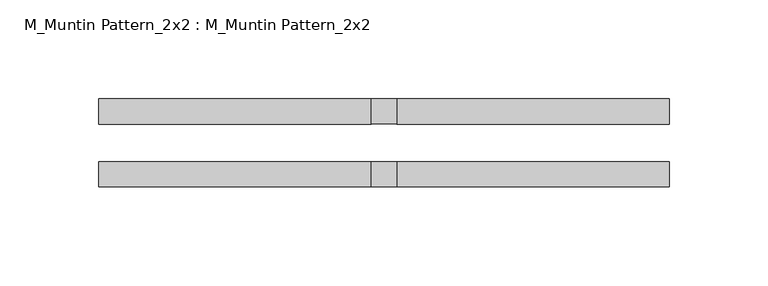
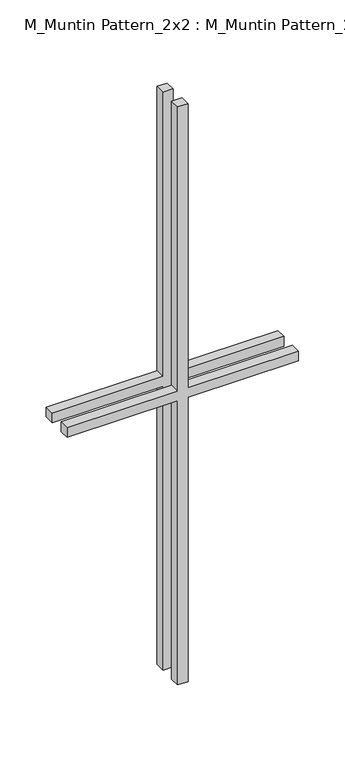
"""IFC4 building model written with IfcOpenShell, lengths in millimetres: proxy geometry, M_Muntin Pattern_2x2 : M_Muntin Pattern_2x2."""

from ifc_helpers import new_model, si_unit, frame, origin, place, context, project, spatial, polyline, outline, extrude, source, transform, mapped, element, save


def m_muntin_pattern_2x2_m_muntin_pattern_2x2_4fd78f17(model_context):
    return source(origin(), model_context, "Body", "SweptSolid", [
        extrude(outline(polyline([(386.5, -6.35), (386.5, -144.2375), (373.8, -144.2375), (373.8, -6.35), (0.0, -6.35), (0.0, 6.35), (373.8, 6.35), (373.8, 144.2375), (386.5, 144.2375), (386.5, 6.35), (760.3, 6.35), (760.3, -6.35), (386.5, -6.35)])), frame((0.0, -22.225, 0.0), z_axis=(0.0, 1.0, 0.0), x_axis=(0.0, 0.0, 1.0)), (0.0, 0.0, 1.0), 12.7),
        extrude(outline(polyline([(386.5, -6.35), (386.5, -144.2375), (373.8, -144.2375), (373.8, -6.35), (0.0, -6.35), (0.0, 6.35), (373.8, 6.35), (373.8, 144.2375), (386.5, 144.2375), (386.5, 6.35), (760.3, 6.35), (760.3, -6.35), (386.5, -6.35)])), frame((0.0, 9.525, 0.0), z_axis=(0.0, 1.0, 0.0), x_axis=(0.0, 0.0, 1.0)), (0.0, 0.0, 1.0), 12.7),
    ])


if __name__ == "__main__":
    model = new_model("IFC4")
    model_context = context("Model", 3, world=origin())
    ifc_project = project(units=[si_unit("LENGTHUNIT", "METRE", prefix="MILLI")], contexts=[model_context])
    site = spatial("IfcSite", under=ifc_project)
    building = spatial("IfcBuilding", under=site)
    placement = place(None, origin())
    m_muntin_pattern_2x2_m_muntin_pattern_2x2_shape = m_muntin_pattern_2x2_m_muntin_pattern_2x2_4fd78f17(model_context)
    element("IfcBuildingElementProxy", 1, Name="M_Muntin Pattern_2x2 : M_Muntin Pattern_2x2", ObjectType="M_Muntin Pattern_2x2 : M_Muntin Pattern_2x2", at=placement, inside=building, context=model_context, shape_type="MappedRepresentation", body=[
        mapped(m_muntin_pattern_2x2_m_muntin_pattern_2x2_shape, transform((0.0, 0.0, 0.0), x_axis=(1.0, 0.0, 0.0), y_axis=(0.0, 1.0, 0.0), z_axis=(0.0, 0.0, 1.0))),
    ])
    save(model, "model.ifc")

# Revit data of these elements
# Type "M_Muntin Pattern_2x2 : M_Muntin Pattern_2x2"
#   Width [instance default] = 1200 mm
#   Thickness = 12.7 mm
#   Height [instance default] = 1200 mm
#   Distance = 19.05 mm
#   Interior Material [instance default] = none
#   Exterior Material [instance default] = none
#   Default Elevation = 0
# Element 1 (IfcBuildingElementProxy, "M_Muntin Pattern_2x2 : M_Muntin Pattern_2x2")
#   Width = 288.475 mm
#   Height = 760.3 mm
#   Interior Material = Wood - Stained
#   Exterior Material = Clad - White
#   Materials on its faces: "Clad - White", "Wood - Stained"
# Materials
#   "Clad - White": class "Wood", colour RGB 242 242 238, transparency 0, Cost = 0
#   "Wood - Stained": class "Wood", colour RGB 224 178 126, transparency 0, Cost = 0
